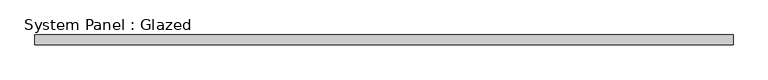
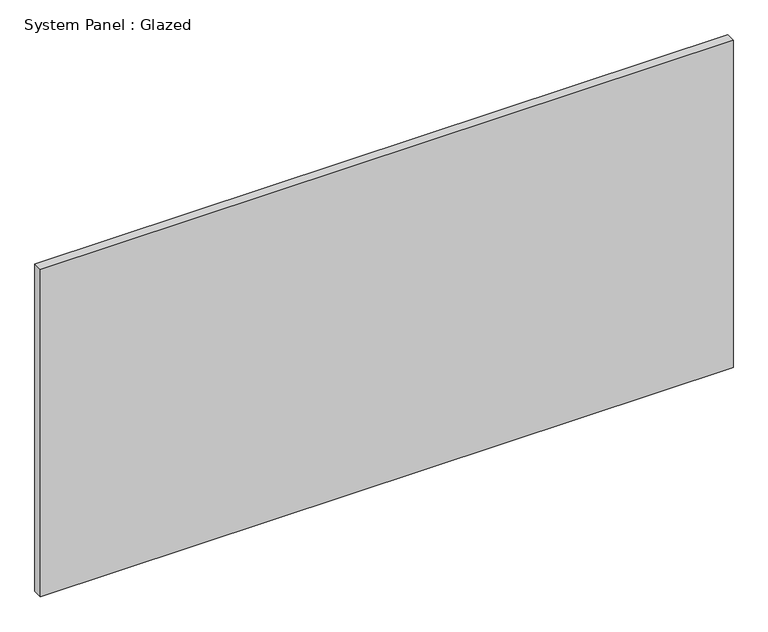
"""IFC4 building model written with IfcOpenShell, lengths in millimetres: plate geometry, System Panel : Glazed."""

from ifc_helpers import new_model, si_unit, origin, origin_with_axes, place, context, project, spatial, polyline, outline, extrude, source, transform, mapped, element, save


def system_panel_glazed_95be5de7(model_context):
    return source(origin(), model_context, "Body", "SweptSolid", [
        extrude(outline(polyline([(914.4, 19.05), (-914.4, 19.05), (-914.4, 44.45), (914.4, 44.45), (914.4, 19.05)])), origin_with_axes(), (0.0, 0.0, 1.0), 914.4),
    ])


if __name__ == "__main__":
    model = new_model("IFC4")
    model_context = context("Model", 3, world=origin())
    ifc_project = project(units=[si_unit("LENGTHUNIT", "METRE", prefix="MILLI")], contexts=[model_context])
    site = spatial("IfcSite", under=ifc_project)
    building = spatial("IfcBuilding", under=site)
    placement = place(None, origin())
    system_panel_glazed_shape = system_panel_glazed_95be5de7(model_context)
    element("IfcPlate", 1, ObjectType="System Panel : Glazed", at=placement, inside=building, context=model_context, shape_type="MappedRepresentation", body=[
        mapped(system_panel_glazed_shape, transform((0.0, 0.0, 0.0), x_axis=(1.0, 0.0, 0.0), y_axis=(0.0, 1.0, 0.0), z_axis=(0.0, 0.0, 1.0))),
    ])
    save(model, "model.ifc")

# Revit data of these elements
# Type "System Panel : Glazed"
#   Construction Type Id = "GSP4R"
#   Analytic Construction = "1/8 in Pilkington single glazing"
#   Visual Light Transmittance = 0.9
#   Solar Heat Gain Coefficient = 0.86
#   Heat Transfer Coefficient (U) = 1.18115 BTU/(h·ft²·°F)
# Element 1 (IfcPlate, "System Panel : Glazed")
#   Materials on its faces: "Glass"
# Materials
#   "Glass": class "Glass", colour RGB 0 128 192, transparency 0.75, Description = "Soda Lime Glass", Cost = 0
